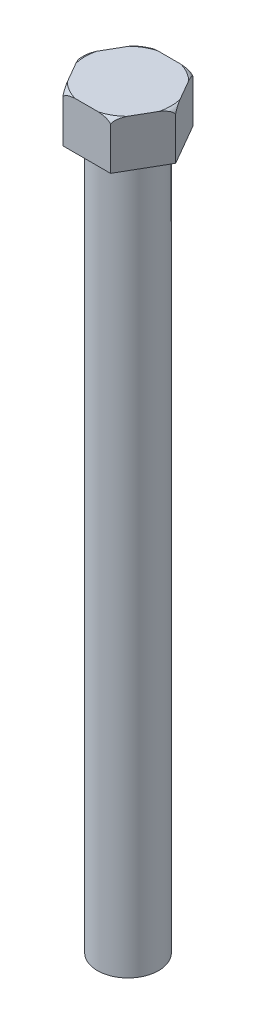
from build123d import *

# Parameters (mm, degrees)
HEX_HEAD_DEPTH     = 20
SHANK_PROFILE_26_R = 13
SHANK_26X300_DEPTH = 300


with BuildPart() as part:
    # Hex Head Profile 35AF → Hex Head (new body)
    with BuildSketch(Plane(origin=(0, 0, 0), x_dir=(1, 0, 0), z_dir=(0, 1, 0))):
        Polygon((20.207259422, 0), (10.103629711, 17.5), (-10.103629711, 17.5), (-20.207259422, 0), (-10.103629711, -17.5), (10.103629711, -17.5), align=None)
    extrude(amount=HEX_HEAD_DEPTH)

    # Shank Profile Ø26 → Shank Ø26x300 (add)
    with BuildSketch(Plane.XZ):
        with Locations(Location((0, 0, 0), (0, 0, 270))):
            Circle(SHANK_PROFILE_26_R)
    extrude(amount=SHANK_26X300_DEPTH)

    # Head Chamfer Profile → Head Chamfer (revolve, cut)
    with BuildSketch(Plane.XY):
        with BuildLine():
            Line((18.207259422, 20), (20.207259422, 20))
            Line((20.207259422, 20), (20.207259422, 18))
            ThreePointArc((20.207259422, 18), (19.457751072, 19.25049165), (18.207259422, 20))
        make_face()
    revolve(axis=Axis((0, 0, 0), (0, 1, 0)), mode=Mode.SUBTRACT)


solid = part.part
